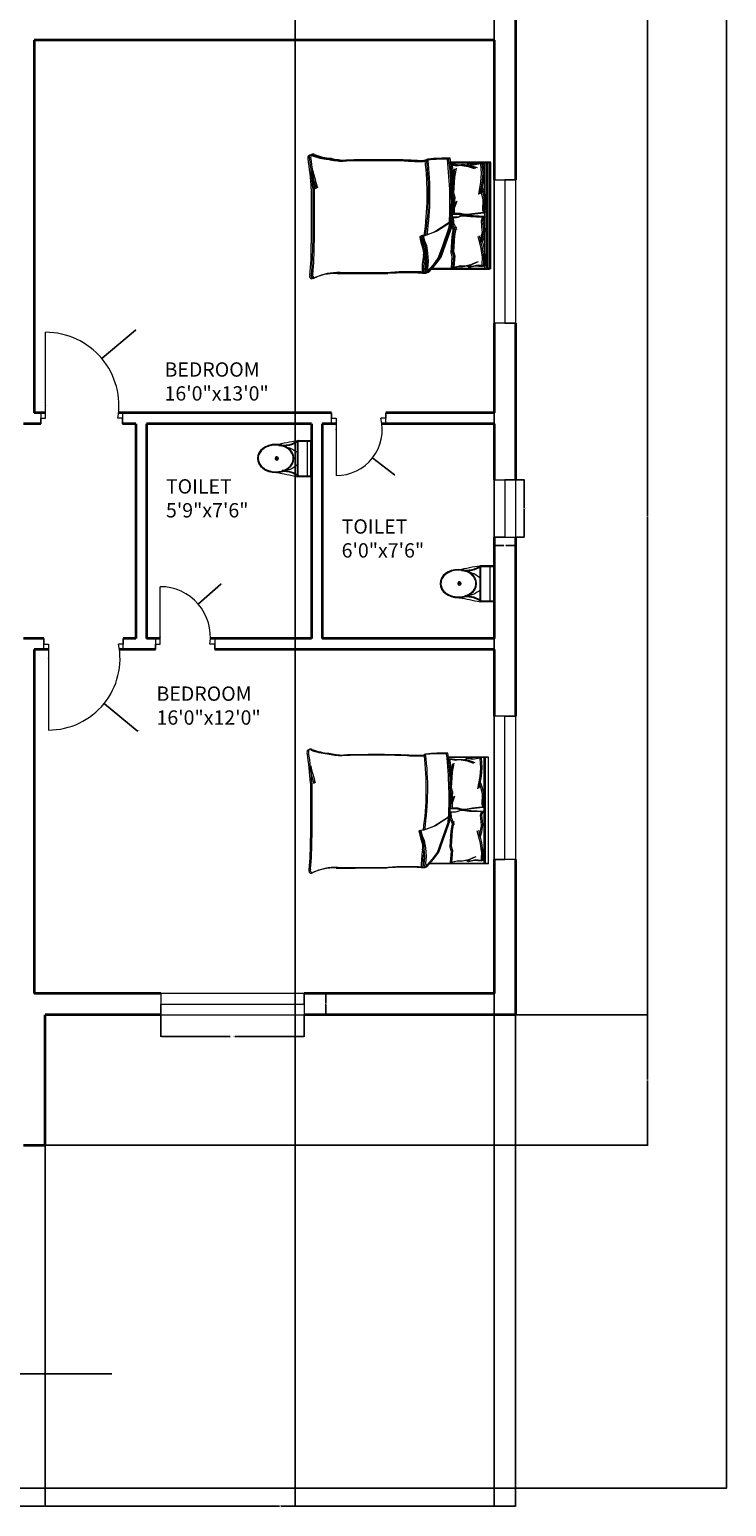
# Model space of a CAD drawing. Units: inches. Extents: x 1902 to 2626, y 1199 to 2408.
# Tile 5 of 9: x 2334 to 2626, y 1199 to 1817. Entities that reach past the tile are written whole.
import ezdxf

# ---------------------------------------------------------------- set-up
doc = ezdxf.new("R2010")
doc.units = ezdxf.units.IN
for name, color, linetype, lineweight in [('A-ANNO-DIMS', 2, 'Continuous', 18), ('A-ANNO-TTLB', 7, 'Continuous', 25), ('A-AREA-IDEN', 7, 'Continuous', 18), ('A-DOOR', 31, 'Continuous', 18), ('A-FLOR-FIXT', 9, 'Continuous', 18), ('A-FURN', 8, 'Continuous', 13), ('A-GLAZ', 181, 'Continuous', 18), ('A-WALL', 7, 'Continuous', 35)]:
    doc.layers.add(name, color=color, linetype=linetype, lineweight=lineweight)
doc.styles.get("Standard").update_dxf_attribs({"font": 'arial.ttf'})
doc.dimstyles.get("Standard").update_dxf_attribs({"dimtxt": 0.18, "dimasz": 0.18, "dimexe": 0.18, "dimexo": 0.0625, "dimgap": 0.09, "dimtad": 0, "dimtih": 1, "dimtoh": 1, "dimdec": 4, "dimzin": 0, "dimdsep": 46, "dimtxsty": 'Standard', "dimcen": 0.09, "dimadec": 0, "dimazin": 0, "dimtfac": 1, "dimtdec": 4, "dimtofl": 0, "dimtmove": 0, "dimatfit": 3, "dimfxl": 1, "dimtolj": 1, "dimtzin": 0, "dimarcsym": 0})

# ---------------------------------------------------------------- blocks, each defined once
blk = doc.blocks.new('A$C31115884')
for p, q in [((283, 498), (223, 498)), ((258, 466), (258, 523)), ((0, 200), (0, 0)), ((520, 200), (0, 200)), ((510, 54), (0, 54)), ((10, 190), (10, 10)), ((510, 190), (10, 190)), ((10, 10), (510, 10)), ((510, 10), (510, 190)), ((520, 0), (520, 200)), ((0, 0), (520, 0))]:
    blk.add_line(p, q)
blk.add_circle((256, 496), 23.6)
for centre, radius, start, end in [((2778, -205), 2807, 165.4549, 171.7133), ((-295, 403), 365, 324.2091, 9.3499), ((-295, 403), 375, 324.2091, 9.3499), ((806, 403), 365, 170.6501, 215.7909), ((3237, 905), 2807, 188.2867, 194.5451), ((384, 406), 293, 190.2774, 224.1564), ((139, 406), 293, 315.8436, 2.6563), ((806, 403), 375, 179.2036, 215.7909)]:
    blk.add_arc(centre, radius, start, end)
blk.add_ellipse((256, 510), major_axis=(0, -261), ratio=0.772727)
blk.add_open_spline([(256, 259), (263, 259), (270, 260), (288, 262), (299, 265), (320, 273), (330, 278), (350, 291), (360, 299), (378, 316), (386, 326), (402, 347), (409, 358), (421, 383), (427, 395), (436, 422), (440, 436), (445, 465), (447, 480), (448, 509), (448, 524), (445, 553), (443, 568), (436, 596), (432, 610), (422, 636), (416, 649), (402, 672), (395, 683), (379, 703), (370, 712), (351, 728), (341, 735), (321, 746), (310, 751), (289, 757), (278, 759), (256, 761), (245, 761), (223, 757), (212, 754), (191, 746), (181, 741), (161, 728), (151, 720), (133, 703), (125, 693), (110, 672), (103, 660), (90, 636), (85, 623), (76, 596), (72, 582), (67, 553), (66, 538), (64, 509), (65, 494), (68, 465), (70, 450), (77, 422), (81, 408), (91, 382), (97, 370), (111, 346), (118, 335), (135, 316), (144, 307), (162, 291), (172, 284), (193, 273), (203, 269), (225, 262), (236, 260), (250, 259), (253, 259), (256, 259)], degree=3, knots=[0, 0, 0, 0, 0.110105, 0.110105, 0.285049, 0.285049, 0.459994, 0.459994, 0.634938, 0.634938, 0.809882, 0.809882, 0.984827, 0.984827, 1.159771, 1.159771, 1.334715, 1.334715, 1.50966, 1.50966, 1.684604, 1.684604, 1.859549, 1.859549, 2.034493, 2.034493, 2.209437, 2.209437, 2.384382, 2.384382, 2.559326, 2.559326, 2.73427, 2.73427, 2.909215, 2.909215, 3.084159, 3.084159, 3.259103, 3.259103, 3.434048, 3.434048, 3.608992, 3.608992, 3.783936, 3.783936, 3.958881, 3.958881, 4.133825, 4.133825, 4.30877, 4.30877, 4.483714, 4.483714, 4.658658, 4.658658, 4.833603, 4.833603, 5.008547, 5.008547, 5.183491, 5.183491, 5.358436, 5.358436, 5.53338, 5.53338, 5.708324, 5.708324, 5.883269, 5.883269, 6.058213, 6.058213, 6.233158, 6.233158, 6.283185, 6.283185, 6.283185, 6.283185])
blk = doc.blocks.new('BED-DOUBLE')
for p, q in [((26.5, 49.58), (23.46, 46.12)), ((26.5, 49.58), (23.46, 46.12)), ((28.13, 49.66), (26.5, 49.58, 3.61)), ((28.13, 49.66), (26.5, 49.58, 3.61)), ((27.08, 48.15), (26.5, 49.58)), ((27.08, 48.15), (26.5, 49.58)), ((-0.01, 48.09), (0.59, 48.09)), ((-0.01, 48.09), (-0.01, 3.46)), ((-0.01, 47.87), (24.84, 47.87)), ((-0.01, 47.87), (24.84, 47.87)), ((0.59, 48.09), (25.44, 48.09)), ((0.59, 48.09), (25.44, 48.09)), ((1.43, 3.25), (1.43, 47.87)), ((1.43, 3.25), (1.43, 47.87)), ((2.02, 3.46), (2.02, 48.09)), ((2.02, 3.46), (2.02, 48.09)), ((2.38, 46.8), (2.29, 41.75)), ((2.38, 46.8), (2.29, 41.75)), ((2.38, 46.8), (5.38, 46.44)), ((2.38, 46.8), (5.38, 46.44)), ((2.98, 47.01), (2.89, 41.97)), ((2.98, 47.01), (2.89, 41.96)), ((2.98, 47.01), (5.98, 46.66)), ((2.98, 47.01), (5.98, 46.66)), ((7.7, 46.05), (5.2, 44.94)), ((7.7, 46.05), (5.2, 44.94)), ((5.38, 46.44), (7.78, 47)), ((5.38, 46.44), (7.78, 47)), ((8.3, 46.26), (5.8, 45.16)), ((8.3, 46.26), (5.8, 45.16)), ((5.98, 46.66), (8.38, 47.21)), ((5.98, 46.66), (8.38, 47.21)), ((11.04, 46.8), (7.7, 46.05)), ((11.04, 46.8), (7.7, 46.05)), ((7.78, 47), (8.76, 46.52)), ((7.78, 47), (8.76, 46.52)), ((11.64, 47.01), (8.3, 46.26)), ((11.64, 47.01), (8.3, 46.26)), ((8.38, 47.21), (9.35, 46.73)), ((8.38, 47.21), (9.35, 46.73)), ((12.54, 46.62), (11.04, 46.8)), ((12.54, 46.62), (11.04, 46.8)), ((13.14, 46.83), (11.64, 47.01)), ((13.14, 46.83), (11.64, 47.01)), ((15.47, 47.34), (12.54, 46.62)), ((15.47, 47.34), (12.54, 46.62)), ((16.07, 47.56), (13.14, 46.83)), ((16.07, 47.56), (13.14, 46.83)), ((15.09, 42.55), (15.47, 47.34)), ((15.09, 42.55), (15.47, 47.34)), ((15.69, 42.77), (16.07, 47.56)), ((15.69, 42.77), (16.07, 47.56)), ((21.44, 43.38), (19.56, 38.17)), ((21.44, 43.38), (19.56, 38.17)), ((22.87, 45.91), (20.84, 43.16)), ((22.87, 45.91), (20.84, 43.16)), ((23.46, 46.12), (21.44, 43.38)), ((23.46, 46.12), (21.44, 43.38)), ((25.9, 49.37), (22.87, 45.91)), ((25.9, 49.37), (22.87, 45.91)), ((27.53, 49.44), (25.9, 49.37, 3.61)), ((27.53, 49.44), (25.9, 49.37, 3.61)), ((26.48, 47.93), (25.9, 49.37)), ((26.48, 47.93), (25.9, 49.37)), ((26.19, 45.04), (26.48, 47.93)), ((26.19, 45.04), (26.48, 47.93)), ((26.48, 41.43), (26.19, 45.04)), ((26.48, 41.43), (26.19, 45.04)), ((26.79, 45.26), (27.08, 48.15)), ((26.79, 45.25), (27.08, 48.15)), ((27.08, 41.64), (26.79, 45.26)), ((27.08, 41.64), (26.79, 45.25)), ((2.29, 41.75), (2.37, 42.69)), ((2.29, 41.75), (2.37, 42.69)), ((2.37, 42.69), (2.86, 39.14)), ((2.37, 42.69), (2.86, 39.14)), ((2.86, 39.14), (4.12, 34.08)), ((2.86, 39.14), (4.12, 34.08)), ((2.89, 41.97), (2.97, 42.9)), ((2.89, 41.96), (2.97, 42.9)), ((2.97, 42.9), (3.46, 39.36)), ((2.97, 42.9), (3.46, 39.35)), ((3.46, 39.36), (4.72, 34.29)), ((3.46, 39.35), (4.72, 34.29)), ((15.61, 40.72), (15.09, 42.55)), ((15.61, 40.72), (15.09, 42.55)), ((15.21, 34.18), (15.61, 40.72)), ((15.21, 34.18), (15.61, 40.72)), ((16.21, 40.93), (15.69, 42.77)), ((16.21, 40.93), (15.69, 42.77)), ((15.81, 34.39), (16.21, 40.93)), ((15.81, 34.39), (16.21, 40.93)), ((18.97, 37.96), (16.23, 30.17)), ((18.97, 37.96), (16.23, 30.17)), ((19.56, 38.17), (16.82, 30.38)), ((19.56, 38.17), (16.82, 30.38)), ((20.84, 43.16), (18.97, 37.96)), ((20.84, 43.16), (18.97, 37.96)), ((26.91, 38.25), (26.48, 41.43)), ((26.91, 38.24), (26.48, 41.43)), ((27.78, 36.37), (26.91, 38.25)), ((27.78, 36.36), (26.91, 38.24)), ((27.51, 38.46), (27.08, 41.64)), ((27.51, 38.46), (27.08, 41.64)), ((28.38, 36.58), (27.51, 38.46)), ((28.38, 36.58), (27.51, 38.46)), ((74.59, 14.28), (74.59, 37.27)), ((74.59, 14.28), (74.59, 37.27)), ((2.87, 34.68), (2.36, 31.94)), ((2.87, 34.68), (2.36, 31.94)), ((2.36, 31.94), (2.38, 31.64)), ((2.36, 31.94), (2.38, 31.64)), ((2.38, 31.64), (2.78, 27.51)), ((2.38, 31.64), (2.78, 27.51)), ((3.42, 36.61), (2.87, 34.68)), ((3.42, 36.61), (2.87, 34.68)), ((3.47, 34.89), (2.96, 32.16)), ((3.47, 34.89), (2.96, 32.16)), ((2.96, 32.16), (2.98, 31.86)), ((2.96, 32.16), (2.98, 31.86)), ((2.98, 31.86), (3.37, 27.72)), ((2.98, 31.86), (3.37, 27.72)), ((4.02, 36.82), (3.47, 34.89)), ((4.02, 36.82), (3.47, 34.89)), ((15.63, 28.72), (14.43, 31.58)), ((15.63, 28.72), (14.43, 31.58)), ((14.59, 30.41), (15.21, 34.18)), ((14.59, 30.41), (15.21, 34.18)), ((16.22, 28.93), (15.02, 31.8)), ((16.22, 28.93), (15.02, 31.8)), ((15.18, 30.62), (15.81, 34.39)), ((15.18, 30.62), (15.81, 34.39)), ((16.23, 28.26), (22.29, 32.17)), ((16.23, 28.26), (22.29, 32.17)), ((16.82, 28.47), (22.89, 32.38)), ((16.82, 28.47), (22.89, 32.38)), ((22.29, 32.17), (26.48, 33.76)), ((22.29, 32.17), (26.48, 33.76)), ((22.89, 32.38), (27.08, 33.98)), ((22.89, 32.38), (27.08, 33.98)), ((26.48, 33.76), (28.36, 34.05)), ((26.48, 33.76), (28.36, 34.05)), ((27.08, 33.98), (28.96, 34.26)), ((27.08, 33.98), (28.96, 34.26)), ((28.36, 34.05), (27.78, 36.37)), ((28.36, 34.05), (27.78, 36.36)), ((28.96, 34.26), (28.38, 36.58)), ((28.96, 34.26), (28.38, 36.58)), ((73.99, 14.07), (73.99, 37.05)), ((73.99, 14.07), (73.99, 37.05)), ((1.74, 24.27), (6.74, 24.81)), ((1.74, 24.27), (6.74, 24.81)), ((2.78, 27.51), (2.32, 26.13)), ((2.78, 27.51), (2.32, 26.13)), ((2.32, 26.13), (7.34, 25.9)), ((2.32, 26.13), (7.34, 25.9)), ((2.34, 24.48), (7.33, 25.02)), ((2.34, 24.48), (7.33, 25.02)), ((3.37, 27.72), (2.92, 26.34)), ((3.37, 27.72), (2.92, 26.34)), ((2.92, 26.34), (7.94, 26.11)), ((2.92, 26.34), (7.94, 26.11)), ((6.74, 24.81), (9.71, 25.35)), ((6.74, 24.81), (9.71, 25.35)), ((7.33, 25.02), (10.3, 25.56)), ((7.33, 25.02), (10.3, 25.56)), ((7.34, 25.9), (10.34, 25.55)), ((7.34, 25.9), (10.34, 25.55)), ((7.94, 26.11), (10.94, 25.76)), ((7.94, 26.11), (10.94, 25.76)), ((9.71, 25.35), (10.92, 25.35)), ((9.71, 25.35), (10.92, 25.35)), ((10.3, 25.56), (11.52, 25.56)), ((10.3, 25.56), (11.52, 25.56)), ((10.34, 25.55), (11.55, 25.62)), ((10.34, 25.55), (11.55, 25.62)), ((10.92, 25.35), (12.68, 24.81)), ((10.92, 25.35), (12.68, 24.81)), ((10.94, 25.76), (12.15, 25.84)), ((10.94, 25.76), (12.15, 25.84)), ((11.52, 25.56), (13.27, 25.02)), ((11.52, 25.56), (13.27, 25.02)), ((11.55, 25.62), (13.27, 26.27)), ((11.55, 25.62), (13.27, 26.27)), ((12.15, 25.84), (13.87, 26.48)), ((12.15, 25.84), (13.87, 26.48)), ((12.68, 24.81), (15.18, 24.81)), ((12.68, 24.81), (15.18, 24.81)), ((13.27, 26.27), (15.77, 26.43)), ((13.27, 26.27), (15.77, 26.43)), ((13.27, 25.02), (15.78, 25.02)), ((13.27, 25.02), (15.78, 25.02)), ((13.87, 26.48), (16.37, 26.64)), ((13.87, 26.48), (16.37, 26.64)), ((15.18, 24.81), (15.18, 22.51)), ((15.18, 24.81), (15.18, 22.51)), ((15.77, 26.43), (15.63, 28.72)), ((15.77, 26.43), (15.63, 28.72)), ((15.78, 25.02), (15.78, 22.72)), ((15.78, 25.02), (15.78, 22.72)), ((16.37, 26.64), (16.22, 28.93)), ((16.37, 26.64), (16.22, 28.93)), ((2.28, 22.92), (1.74, 24.27)), ((2.28, 22.92), (1.74, 24.27)), ((2.15, 18.76), (2.28, 22.92)), ((2.15, 18.76), (2.28, 22.92)), ((2.15, 18.46), (2.15, 18.76)), ((2.15, 18.46), (2.15, 18.76)), ((2.88, 23.13), (2.34, 24.48)), ((2.88, 23.13), (2.34, 24.48)), ((2.74, 18.98), (2.88, 23.13)), ((2.74, 18.98), (2.88, 23.13)), ((2.74, 18.68), (2.74, 18.98)), ((2.74, 18.68), (2.74, 18.98)), ((3.42, 15.98), (2.74, 18.68)), ((3.42, 15.98), (2.74, 18.68)), ((15.18, 22.51), (14.16, 19.57)), ((15.18, 22.51), (14.16, 19.57)), ((15.78, 22.72), (14.76, 19.79)), ((15.78, 22.72), (14.76, 19.79)), ((15.09, 18.1), (15.47, 22.9)), ((15.09, 18.1), (15.47, 22.9)), ((15.69, 18.32), (16.07, 23.11)), ((15.69, 18.32), (16.07, 23.11)), ((2.82, 15.76), (2.15, 18.46)), ((2.82, 15.76), (2.15, 18.46)), ((3.5, 13.88), (2.82, 15.76)), ((3.5, 13.87), (2.82, 15.76)), ((3.09, 11.31), (4.04, 16.44)), ((3.09, 11.31), (4.04, 16.44)), ((4.09, 14.09), (3.42, 15.98)), ((4.09, 14.09), (3.42, 15.98)), ((3.69, 11.52), (4.63, 16.65)), ((3.69, 11.52), (4.63, 16.65)), ((15.61, 16.27), (15.09, 18.1)), ((15.61, 16.27), (15.09, 18.1)), ((15.21, 9.73), (15.61, 16.27)), ((15.21, 9.73), (15.61, 16.27)), ((16.21, 16.49), (15.69, 18.32)), ((16.21, 16.49), (15.69, 18.32)), ((15.81, 9.94), (16.21, 16.49)), ((15.81, 9.94), (16.21, 16.49)), ((2.8, 7.64), (2.82, 7.74)), ((2.8, 7.64), (2.82, 7.74)), ((3.11, 3.64), (2.8, 7.64)), ((3.11, 3.64), (2.8, 7.64)), ((2.82, 7.74), (3.09, 11.31)), ((2.82, 7.74), (3.09, 11.31)), ((3.4, 7.86), (3.42, 7.95)), ((3.4, 7.86), (3.42, 7.95)), ((3.71, 3.86), (3.4, 7.86)), ((3.71, 3.86), (3.4, 7.86)), ((3.42, 7.95), (3.69, 11.52)), ((3.42, 7.95), (3.69, 11.52)), ((14.59, 5.96), (15.21, 9.73)), ((14.59, 5.96), (15.21, 9.73)), ((15.18, 6.18), (15.81, 9.94)), ((15.18, 6.18), (15.81, 9.94)), ((15.21, 9.73), (15.51, 8.67)), ((15.21, 9.73), (15.51, 8.67)), ((15.51, 8.67), (16.19, 3.91)), ((15.51, 8.67), (16.19, 3.91)), ((15.81, 9.94), (16.11, 8.88)), ((15.81, 9.94), (16.11, 8.88)), ((16.11, 8.88), (16.78, 4.12)), ((16.11, 8.88), (16.78, 4.12)), ((16.91, 3.25), (-0.01, 3.25)), ((16.91, 3.25), (-0.01, 3.25)), ((17.5, 3.46), (0.59, 3.46)), ((17.5, 3.46), (0.59, 3.46)), ((3.09, 3.64), (6.06, 4.18)), ((3.09, 3.64), (6.06, 4.18)), ((3.69, 3.85), (6.66, 4.39)), ((3.69, 3.85), (6.66, 4.39)), ((8.36, 4.72), (5.79, 5.67)), ((8.36, 4.72), (5.79, 5.67)), ((6.06, 4.18), (8.49, 3.78)), ((6.06, 4.18), (8.49, 3.78)), ((8.95, 4.93), (6.39, 5.88)), ((8.95, 4.93), (6.39, 5.88)), ((6.66, 4.39), (9.09, 3.99)), ((6.66, 4.39), (9.09, 3.99)), ((11.73, 4.18), (8.36, 4.72)), ((11.73, 4.18), (8.36, 4.72)), ((8.49, 3.78), (9.44, 4.32)), ((8.49, 3.78), (9.44, 4.32)), ((12.33, 4.39), (8.95, 4.93)), ((12.33, 4.39), (8.95, 4.93)), ((9.09, 3.99), (10.03, 4.53)), ((9.09, 3.99), (10.03, 4.53)), ((13.22, 4.45), (11.73, 4.18)), ((13.22, 4.45), (11.73, 4.18)), ((13.81, 4.66), (12.33, 4.39)), ((13.81, 4.66), (12.33, 4.39)), ((16.19, 3.91), (13.22, 4.45)), ((16.19, 3.91), (13.22, 4.45)), ((16.78, 4.12), (13.81, 4.66)), ((16.78, 4.12), (13.81, 4.66))]:
    blk.add_line(p, q)
for centre, radius, start, end in [((33.9, 170.19), 120.92, 266.97912, 273.83645), ((33.9, 170.19), 120.92, 266.97912, 273.83645), ((-5.62, 48.14), 33.79, 349.87628, 2.56571), ((-5.62, 48.14), 33.79, 349.87628, 2.56571), ((34.5, 170.41), 120.92, 266.97912, 273.83645), ((34.5, 170.41), 120.92, 266.97912, 273.83645), ((63.32, -4210.02), 4259.62, 90.00217, 90.28689), ((63.32, -4210.02), 4259.62, 90.00217, 90.28689), ((63.92, -4209.8), 4259.62, 90.00217, 90.28689), ((63.92, -4209.8), 4259.62, 90.00217, 90.28689), ((64.11, 71.12), 21.54, 267.47136, 296.46809), ((64.11, 71.12), 21.54, 267.47136, 296.46809), ((64.71, 71.33), 21.54, 267.47136, 296.46809), ((64.71, 71.33), 21.54, 267.47136, 296.46809), ((73.64, 50.81), 1.03, 332.65876, 86.02002), ((73.64, 50.81), 1.03, 332.65876, 86.02002), ((198.21, 38.43), 124.23, 174.4998, 180.63509), ((198.21, 38.43), 124.23, 174.4998, 180.63509), ((74.24, 51.02), 1.03, 332.65876, 86.02002), ((74.24, 51.02), 1.03, 332.65876, 86.02002), ((198.8, 38.64), 124.23, 174.4998, 180.63509), ((198.8, 38.64), 124.23, 174.4998, 180.63509), ((-6.22, 47.93), 33.79, 349.87628, 2.56571), ((-6.22, 47.93), 33.79, 349.87628, 2.56571), ((32.74, 40.85), 5.81, 168.6608, 203.73842), ((32.74, 40.85), 5.81, 168.6608, 203.73842), ((1.38, 29.09), 27.69, 10.66171, 19.88058), ((1.38, 29.09), 27.69, 10.66171, 19.88058), ((33.33, 41.06), 5.81, 168.6608, 203.73842), ((33.33, 41.06), 5.81, 168.6608, 203.73842), ((1.98, 29.31), 27.69, 10.66171, 19.88058), ((1.98, 29.31), 27.69, 10.66171, 19.88058), ((145.95, 16.58), 120.47, 171.78449, 186.90062), ((145.95, 16.58), 120.47, 171.78449, 186.90062), ((146.55, 16.8), 120.47, 171.78449, 186.90062), ((146.55, 16.8), 120.47, 171.78449, 186.90062), ((28.42, 34.21), 0.172, 250.24637, 1.13765), ((28.42, 34.21), 0.172, 250.24637, 1.13765), ((29.01, 34.43), 0.172, 250.24637, 1.13765), ((29.01, 34.43), 0.172, 250.24637, 1.13765), ((169.99, 19.95), 154.04, 176.08655, 186.78213), ((169.99, 19.95), 154.04, 176.08655, 186.78213), ((170.58, 20.16), 154.04, 176.08655, 186.78213), ((170.58, 20.16), 154.04, 176.08655, 186.78213), ((-22.15, -16.08), 99.41, 13.38322, 17.70533), ((-22.15, -16.08), 99.41, 13.38322, 17.70533), ((-21.55, -15.86), 99.41, 13.38322, 17.70533), ((-21.55, -15.86), 99.41, 13.38322, 17.70533), ((187.53, 20.01), 113.69, 182.99578, 189.40907), ((187.53, 20.01), 113.69, 182.99578, 189.40907), ((188.12, 20.22), 113.69, 182.99578, 189.40907), ((188.12, 20.22), 113.69, 182.99578, 189.40907), ((18.76, 79.52), 77.79, 268.72178, 275.60397), ((18.76, 79.52), 77.79, 268.72178, 275.60397), ((19.36, 79.74), 77.79, 268.72178, 275.60397), ((19.36, 79.74), 77.79, 268.72178, 275.60397), ((29.1, -156.22), 158.84, 88.4762, 91.00819), ((29.1, -156.22), 158.84, 88.4762, 91.00819), ((29.7, -156), 158.84, 88.4762, 91.00819), ((29.7, -156.01), 158.84, 88.4762, 91.00819), ((47.26, 452.71), 450.36, 268.22771, 271.71854), ((47.26, 452.71), 450.36, 268.22771, 271.71854), ((47.85, 452.92), 450.36, 268.22771, 271.71854), ((47.85, 452.92), 450.36, 268.22771, 271.71854), ((60.24, -25.11), 27.67, 76.06484, 88.91125), ((60.24, -25.11), 27.67, 76.06484, 88.91125), ((60.83, -24.9), 27.67, 76.06484, 88.91125), ((60.83, -24.9), 27.67, 76.06484, 88.91125), ((65.61, -20.22), 22, 67.97508, 86.652), ((65.61, -20.22), 22, 67.97508, 86.652), ((66.21, -20.01), 22, 67.97508, 86.652), ((66.21, -20.01), 22, 67.97508, 86.652), ((74.43, 1.02), 1.02, 236.17358, 23.47814), ((74.43, 1.02), 1.02, 236.17358, 23.47814), ((75.03, 1.23), 1.02, 236.17358, 23.47814), ((75.03, 1.23), 1.02, 236.17358, 23.47814)]:
    blk.add_arc(centre, radius, start, end)
blk = doc.blocks.new('WINDOW-60-A')
for p, q in [((0, 9), (0, 0)), ((60, 9), (0, 9)), ((60, 4.5), (60, 9)), ((60, 9), (60, 0)), ((0, 0), (0, 4.5)), ((0, 4.5), (60, 4.5)), ((0, 0), (60, 0))]:
    blk.add_line(p, q)
blk = doc.blocks.new('WINDOW-60-B')
for p, q in [((0, 60), (9, 60)), ((0, 60), (0, 0)), ((9, 60), (4.5, 60)), ((4.5, 60), (4.5, 0)), ((9, 60), (9, 0)), ((9, 0), (0, 0)), ((4.5, 0), (9, 0))]:
    blk.add_line(p, q)
blk = doc.blocks.new('WINDOW-24')
for p, q in [((0, 24), (9, 24)), ((0, 24), (0, 0)), ((9, 24), (4.5, 24)), ((4.5, 24), (4.5, 0)), ((9, 24), (9, 0)), ((4.5, 0), (0, 0)), ((0, 0), (9, 0))]:
    blk.add_line(p, q)
blk = doc.blocks.new('*D16')
at = {"layer": 'A-ANNO-DIMS', "color": 0, "lineweight": -2, "transparency": 16777216}
for p, q in [((2389.37, 1404.41), (2389.37, 1395.29)), ((2449.37, 1404.41), (2449.37, 1395.29)), ((2389.55, 1395.47), (2418.41, 1395.47)), ((2449.19, 1395.47), (2420.34, 1395.47))]:
    blk.add_line(p, q, dxfattribs=at)
at = {"layer": 'A-ANNO-DIMS', "color": 0, "transparency": 16777216}
for points in [[(2389.55, 1395.5), (2389.55, 1395.44), (2389.37, 1395.47)], [(2449.19, 1395.5), (2449.19, 1395.44), (2449.37, 1395.47)]]:
    blk.add_solid(points, dxfattribs=at)
at = {"layer": 'Defpoints', "color": 0, "transparency": 16777216}
for p in [(2389.37, 1404.47), (2449.37, 1404.47), (2449.37, 1395.47)]:
    blk.add_point(p, dxfattribs=at)
at = {"layer": 'A-ANNO-DIMS', "color": 0, "transparency": 16777216, "insert": (2419.37, 1395.47), "char_height": 0.18, "attachment_point": 5}
blk.add_mtext('\\A1;WIN. A 60 TYP.', dxfattribs=at)
blk = doc.blocks.new('*D17')
at = {"layer": 'A-ANNO-DIMS', "color": 0, "lineweight": -2, "transparency": 16777216}
for p, q in [((2449.44, 1413.47), (2458.55, 1413.47)), ((2458.37, 1413.29), (2458.37, 1409.16)), ((2449.44, 1404.47), (2458.55, 1404.47)), ((2458.37, 1404.65), (2458.37, 1408.79))]:
    blk.add_line(p, q, dxfattribs=at)
at = {"layer": 'A-ANNO-DIMS', "color": 0, "transparency": 16777216}
for points in [[(2458.34, 1413.29), (2458.4, 1413.29), (2458.37, 1413.47)], [(2458.34, 1404.65), (2458.4, 1404.65), (2458.37, 1404.47)]]:
    blk.add_solid(points, dxfattribs=at)
at = {"layer": 'Defpoints', "color": 0, "transparency": 16777216}
for p in [(2449.37, 1413.47), (2458.37, 1413.47), (2449.37, 1404.47)]:
    blk.add_point(p, dxfattribs=at)
at = {"layer": 'A-ANNO-DIMS', "color": 0, "transparency": 16777216, "insert": (2458.37, 1408.97), "char_height": 0.18, "attachment_point": 5}
blk.add_mtext('\\A1;9 TYP.', dxfattribs=at)
blk = doc.blocks.new('*D20')
at = {"layer": 'A-ANNO-DIMS', "color": 0, "lineweight": -2, "transparency": 16777216}
for p, q in [((2537.91, 1628.52), (2541.63, 1628.52)), ((2541.45, 1628.34), (2541.45, 1616.71)), ((2541.45, 1604.7), (2541.45, 1616.34)), ((2537.91, 1604.52), (2541.63, 1604.52))]:
    blk.add_line(p, q, dxfattribs=at)
at = {"layer": 'A-ANNO-DIMS', "color": 0, "transparency": 16777216}
for points in [[(2541.42, 1628.34), (2541.48, 1628.34), (2541.45, 1628.52)], [(2541.42, 1604.7), (2541.48, 1604.7), (2541.45, 1604.52)]]:
    blk.add_solid(points, dxfattribs=at)
at = {"layer": 'Defpoints', "color": 0, "transparency": 16777216}
for p in [(2537.85, 1628.52), (2541.45, 1628.52), (2537.85, 1604.52)]:
    blk.add_point(p, dxfattribs=at)
at = {"layer": 'A-ANNO-DIMS', "color": 0, "transparency": 16777216, "insert": (2541.45, 1616.52), "char_height": 0.18, "attachment_point": 5}
blk.add_mtext('\\A1;WIN. C 24 TYP.', dxfattribs=at)
blk = doc.blocks.new('*D21')
at = {"layer": 'A-ANNO-DIMS', "color": 0, "lineweight": -2, "transparency": 16777216}
for p, q in [((2528.85, 1604.46), (2528.85, 1600.74)), ((2537.85, 1604.46), (2537.85, 1600.74)), ((2529.03, 1600.92), (2532.89, 1600.92)), ((2537.67, 1600.92), (2533.81, 1600.92))]:
    blk.add_line(p, q, dxfattribs=at)
at = {"layer": 'A-ANNO-DIMS', "color": 0, "transparency": 16777216}
for points in [[(2529.03, 1600.95), (2529.03, 1600.89), (2528.85, 1600.92)], [(2537.67, 1600.95), (2537.67, 1600.89), (2537.85, 1600.92)]]:
    blk.add_solid(points, dxfattribs=at)
at = {"layer": 'Defpoints', "color": 0, "transparency": 16777216}
for p in [(2528.85, 1604.52), (2537.85, 1604.52), (2537.85, 1600.92)]:
    blk.add_point(p, dxfattribs=at)
at = {"layer": 'A-ANNO-DIMS', "color": 0, "transparency": 16777216, "insert": (2533.35, 1600.92), "char_height": 0.18, "attachment_point": 5}
blk.add_mtext('\\A1;9 TYP.', dxfattribs=at)
blk = doc.blocks.new('*D31')
at = {"layer": 'A-ANNO-DIMS', "color": 0, "lineweight": -2, "transparency": 16777216}
for p, q in [((2202.85, 1349.87), (2202.85, 1198.67)), ((2340.85, 1349.87), (2340.85, 1198.67)), ((2203.03, 1198.85), (2271.57, 1198.85)), ((2340.67, 1198.85), (2272.13, 1198.85))]:
    blk.add_line(p, q, dxfattribs=at)
at = {"layer": 'A-ANNO-DIMS', "color": 0, "transparency": 16777216}
for points in [[(2203.03, 1198.88), (2203.03, 1198.82), (2202.85, 1198.85)], [(2340.67, 1198.88), (2340.67, 1198.82), (2340.85, 1198.85)]]:
    blk.add_solid(points, dxfattribs=at)
at = {"layer": 'Defpoints', "color": 0, "transparency": 16777216}
for p in [(2202.85, 1349.93), (2340.85, 1349.93), (2340.85, 1198.85)]:
    blk.add_point(p, dxfattribs=at)
at = {"layer": 'A-ANNO-DIMS', "color": 0, "transparency": 16777216, "insert": (2271.85, 1198.85), "char_height": 0.18, "attachment_point": 5}
blk.add_mtext('\\A1;138', dxfattribs=at)
blk = doc.blocks.new('*D32')
at = {"layer": 'A-ANNO-DIMS', "color": 0, "lineweight": -2, "transparency": 16777216}
for p, q in [((2537.85, 1404.41), (2537.85, 1198.67)), ((2340.85, 1349.87), (2340.85, 1198.67)), ((2341.03, 1198.85), (2439.07, 1198.85)), ((2537.67, 1198.85), (2439.63, 1198.85))]:
    blk.add_line(p, q, dxfattribs=at)
at = {"layer": 'A-ANNO-DIMS', "color": 0, "transparency": 16777216}
for points in [[(2341.03, 1198.88), (2341.03, 1198.82), (2340.85, 1198.85)], [(2537.67, 1198.88), (2537.67, 1198.82), (2537.85, 1198.85)]]:
    blk.add_solid(points, dxfattribs=at)
at = {"layer": 'Defpoints', "color": 0, "transparency": 16777216}
for p in [(2537.85, 1404.47), (2340.85, 1349.93), (2537.85, 1198.85)]:
    blk.add_point(p, dxfattribs=at)
at = {"layer": 'A-ANNO-DIMS', "color": 0, "transparency": 16777216, "insert": (2439.35, 1198.85), "char_height": 0.18, "attachment_point": 5}
blk.add_mtext('\\A1;197', dxfattribs=at)
blk = doc.blocks.new('*D34')
at = {"layer": 'A-ANNO-DIMS', "color": 0, "lineweight": -2, "transparency": 16777216}
for p, q in [((2528.91, 1821.47), (2593.33, 1821.47)), ((2593.15, 1821.29), (2593.15, 1613.15)), ((2593.15, 1404.65), (2593.15, 1612.79)), ((2537.91, 1404.47), (2593.33, 1404.47))]:
    blk.add_line(p, q, dxfattribs=at)
at = {"layer": 'A-ANNO-DIMS', "color": 0, "transparency": 16777216}
for points in [[(2593.12, 1821.29), (2593.18, 1821.29), (2593.15, 1821.47)], [(2593.12, 1404.65), (2593.18, 1404.65), (2593.15, 1404.47)]]:
    blk.add_solid(points, dxfattribs=at)
at = {"layer": 'Defpoints', "color": 0, "transparency": 16777216}
for p in [(2528.85, 1821.47), (2593.15, 1821.47), (2537.85, 1404.47)]:
    blk.add_point(p, dxfattribs=at)
at = {"layer": 'A-ANNO-DIMS', "color": 0, "transparency": 16777216, "insert": (2593.15, 1612.97), "char_height": 0.18, "attachment_point": 5}
blk.add_mtext('\\A1;417', dxfattribs=at)
blk = doc.blocks.new('*D36')
at = {"layer": 'A-ANNO-DIMS', "color": 0, "lineweight": -2, "transparency": 16777216}
for p, q in [((2537.91, 1404.47), (2593.33, 1404.47)), ((2593.15, 1404.29), (2593.15, 1377.38)), ((2593.15, 1350.11), (2593.15, 1377.02)), ((2340.91, 1349.93), (2593.33, 1349.93))]:
    blk.add_line(p, q, dxfattribs=at)
at = {"layer": 'A-ANNO-DIMS', "color": 0, "transparency": 16777216}
for points in [[(2593.12, 1404.29), (2593.18, 1404.29), (2593.15, 1404.47)], [(2593.12, 1350.11), (2593.18, 1350.11), (2593.15, 1349.93)]]:
    blk.add_solid(points, dxfattribs=at)
at = {"layer": 'Defpoints', "color": 0, "transparency": 16777216}
for p in [(2537.85, 1404.47), (2593.15, 1404.47), (2340.85, 1349.93)]:
    blk.add_point(p, dxfattribs=at)
at = {"layer": 'A-ANNO-DIMS', "color": 0, "transparency": 16777216, "insert": (2593.15, 1377.2), "char_height": 0.18, "attachment_point": 5}
blk.add_mtext('\\A1;54.54', dxfattribs=at)
blk = doc.blocks.new('*D37')
at = {"layer": 'A-ANNO-DIMS', "color": 0, "lineweight": -2, "transparency": 16777216}
for p, q in [((2445.52, 2280.41), (2445.52, 1198.67)), ((2528.85, 2280.41), (2528.85, 1198.67)), ((2445.7, 1198.85), (2486.79, 1198.85)), ((2528.67, 1198.85), (2487.58, 1198.85))]:
    blk.add_line(p, q, dxfattribs=at)
at = {"layer": 'A-ANNO-DIMS', "color": 0, "transparency": 16777216}
for points in [[(2445.7, 1198.88), (2445.7, 1198.82), (2445.52, 1198.85)], [(2528.67, 1198.88), (2528.67, 1198.82), (2528.85, 1198.85)]]:
    blk.add_solid(points, dxfattribs=at)
at = {"layer": 'Defpoints', "color": 0, "transparency": 16777216}
for p in [(2445.52, 2280.47), (2528.85, 2280.47), (2528.85, 1198.85)]:
    blk.add_point(p, dxfattribs=at)
at = {"layer": 'A-ANNO-DIMS', "color": 0, "transparency": 16777216, "insert": (2487.18, 1198.85), "char_height": 0.18, "attachment_point": 5}
blk.add_mtext('\\A1;83.33', dxfattribs=at)
blk = doc.blocks.new('*D47')
at = {"layer": 'A-ANNO-DIMS', "color": 0, "lineweight": -2, "transparency": 16777216}
for p, q in [((2378.7, 1691.12), (2364.73, 1679.38)), ((2378.88, 1691.12), (2378.7, 1691.12)), ((2341, 1659.52), (2341.18, 1659.52)), ((2341.09, 1659.43), (2341.09, 1659.61))]:
    blk.add_line(p, q, dxfattribs=at)
at = {"layer": 'A-ANNO-DIMS', "color": 0, "transparency": 16777216}
blk.add_solid([(2364.71, 1679.41), (2364.75, 1679.36), (2364.59, 1679.27)], dxfattribs=at)
at = {"layer": 'Defpoints', "color": 0, "transparency": 16777216}
for p in [(2364.59, 1679.27), (2341.09, 1659.52)]:
    blk.add_point(p, dxfattribs=at)
at = {"layer": 'A-ANNO-DIMS', "color": 0, "transparency": 16777216, "insert": (2379.29, 1691.12), "char_height": 0.18, "attachment_point": 5}
blk.add_mtext('\\A1;R30.7', dxfattribs=at)
blk = doc.blocks.new('*D48')
at = {"layer": 'A-ANNO-DIMS', "color": 0, "lineweight": -2, "transparency": 16777216}
for p, q in [((2342.25, 1553.63), (2342.43, 1553.63)), ((2342.34, 1553.54), (2342.34, 1553.72)), ((2379.46, 1523.44), (2365.68, 1534.65)), ((2379.64, 1523.44), (2379.46, 1523.44))]:
    blk.add_line(p, q, dxfattribs=at)
at = {"layer": 'A-ANNO-DIMS', "color": 0, "transparency": 16777216}
blk.add_solid([(2365.7, 1534.67), (2365.66, 1534.62), (2365.54, 1534.76)], dxfattribs=at)
at = {"layer": 'Defpoints', "color": 0, "transparency": 16777216}
for p in [(2342.34, 1553.63), (2365.54, 1534.76)]:
    blk.add_point(p, dxfattribs=at)
at = {"layer": 'A-ANNO-DIMS', "color": 0, "transparency": 16777216, "insert": (2380.19, 1523.44), "char_height": 0.18, "attachment_point": 5}
blk.add_mtext('\\A1;R29.906', dxfattribs=at)
blk = doc.blocks.new('*D53')
at = {"layer": 'A-ANNO-DIMS', "color": 0, "lineweight": -2, "transparency": 16777216}
for p, q in [((2414.48, 1584.78), (2405.08, 1576.6)), ((2414.66, 1584.78), (2414.48, 1584.78)), ((2388.95, 1562.65), (2389.13, 1562.65)), ((2389.04, 1562.56), (2389.04, 1562.74))]:
    blk.add_line(p, q, dxfattribs=at)
at = {"layer": 'A-ANNO-DIMS', "color": 0, "transparency": 16777216}
blk.add_solid([(2405.06, 1576.62), (2405.1, 1576.57), (2404.94, 1576.48)], dxfattribs=at)
at = {"layer": 'Defpoints', "color": 0, "transparency": 16777216}
for p in [(2404.94, 1576.48), (2389.04, 1562.65)]:
    blk.add_point(p, dxfattribs=at)
at = {"layer": 'A-ANNO-DIMS', "color": 0, "transparency": 16777216, "insert": (2415.21, 1584.78), "char_height": 0.18, "attachment_point": 5}
blk.add_mtext('\\A1;R21.077', dxfattribs=at)
blk = doc.blocks.new('*D57')
at = {"layer": 'A-ANNO-DIMS', "color": 0, "lineweight": -2, "transparency": 16777216}
for p, q in [((2462.67, 1649.53), (2462.85, 1649.53)), ((2462.76, 1649.44), (2462.76, 1649.62)), ((2487.11, 1630.53), (2478.12, 1637.54)), ((2487.29, 1630.53), (2487.11, 1630.53))]:
    blk.add_line(p, q, dxfattribs=at)
at = {"layer": 'A-ANNO-DIMS', "color": 0, "transparency": 16777216}
blk.add_solid([(2478.14, 1637.57), (2478.1, 1637.52), (2477.97, 1637.65)], dxfattribs=at)
at = {"layer": 'Defpoints', "color": 0, "transparency": 16777216}
for p in [(2462.76, 1649.53), (2477.97, 1637.65)]:
    blk.add_point(p, dxfattribs=at)
at = {"layer": 'A-ANNO-DIMS', "color": 0, "transparency": 16777216, "insert": (2487.84, 1630.53), "char_height": 0.18, "attachment_point": 5}
blk.add_mtext('\\A1;R19.303', dxfattribs=at)

msp = doc.modelspace()

# ---------------------------------------------------------------- linework, layer by layer
at = {"layer": 'A-ANNO-TTLB'}
msp.add_line((2104.9287, 1254.1475), (2368.8083, 1254.1475), dxfattribs=at)
msp.add_lwpolyline([(1901.6928, 2408.1473), (2626.1646, 2408.1473), (2626.1646, 1206.3103), (1901.6928, 1206.3103)], close=True, dxfattribs=at)
at = {"layer": 'A-DOOR'}
for p, q in [((2341.0862, 1654.2233), (2341.0862, 1690.2233)), ((2339.0862, 1656.4733), (2339.0862, 1651.9733)), ((2339.0862, 1651.9733), (2339.0862, 1654.2233)), ((2339.0862, 1654.2233), (2341.0862, 1654.2233)), ((2339.0862, 1651.9733), (2339.0862, 1651.9733)), ((2373.3259, 1654.2233), (2371.3259, 1654.2233)), ((2373.3259, 1656.4733), (2373.3259, 1651.9733)), ((2373.3259, 1651.9733), (2373.3259, 1654.2233)), ((2460.7554, 1651.9733), (2460.7554, 1656.4733)), ((2460.7554, 1656.4733), (2460.7554, 1654.2233)), ((2460.7554, 1654.2233), (2460.7554, 1654.2233)), ((2460.7554, 1654.2233), (2462.7554, 1654.2233)), ((2462.7554, 1654.2233), (2462.7554, 1630.2233)), ((2483.4786, 1654.2233), (2481.4786, 1654.2233)), ((2483.4786, 1651.9733), (2483.4786, 1656.4733)), ((2483.4786, 1656.4733), (2483.4786, 1654.2233)), ((2389.0386, 1559.7233), (2389.0386, 1583.7233)), ((2340.3371, 1557.4733), (2340.3371, 1561.9733)), ((2340.3371, 1561.9733), (2340.3371, 1559.7233)), ((2340.3371, 1559.7233), (2342.3371, 1559.7233)), ((2342.3371, 1559.7233), (2342.3371, 1523.7233)), ((2373.6154, 1559.7233), (2371.6154, 1559.7233)), ((2373.6154, 1557.4733), (2373.6154, 1561.9733)), ((2373.6154, 1561.9733), (2373.6154, 1559.7233)), ((2387.0386, 1561.9733), (2387.0386, 1557.4733)), ((2387.0386, 1557.4733), (2387.0386, 1559.7233)), ((2387.0386, 1559.7233), (2389.0386, 1559.7233)), ((2411.9122, 1559.7233), (2409.9122, 1559.7233)), ((2411.9122, 1561.9733), (2411.9122, 1557.4733)), ((2411.9122, 1557.4733), (2411.9122, 1559.7233))]:
    msp.add_line(p, q, dxfattribs=at)
for centre, radius, start, end in [((2341.0862, 1659.5228), 30.7005, 350.0598422, 90), ((2462.7554, 1649.5267), 19.3033, 270, 14.0818678), ((2389.0386, 1562.6461), 21.0772, 352.029104, 90), ((2342.3371, 1553.6292), 29.9058, 270, 11.7579684)]:
    msp.add_arc(centre, radius, start, end, dxfattribs=at)
at = {"layer": 'A-WALL'}
for p, q in [((2537.8507, 1865.0569), (2537.8507, 1754.0445)), ((2528.8507, 1812.4733), (2336.3507, 1812.4733)), ((2336.3507, 1812.4733), (2336.3507, 1656.4733)), ((2528.8507, 1812.4733), (2528.8507, 1754.0445)), ((2528.8507, 1694.0445), (2528.8507, 1656.4733)), ((2537.8507, 1694.0445), (2537.8507, 1628.5226)), ((2339.0862, 1651.9733), (2331.8507, 1651.9733)), ((2341.0862, 1656.4733), (2336.3507, 1656.4733)), ((2460.7554, 1656.4733), (2371.6349, 1656.4733)), ((2378.8507, 1651.9733), (2373.3259, 1651.9733)), ((2378.8507, 1651.9733), (2378.8507, 1561.9733)), ((2383.3507, 1651.9733), (2383.3507, 1561.9733)), ((2452.3507, 1651.9733), (2383.3507, 1651.9733)), ((2452.3507, 1651.9733), (2452.3507, 1561.9733)), ((2456.8507, 1651.9733), (2456.8507, 1561.9733)), ((2462.7554, 1651.9733), (2456.8507, 1651.9733)), ((2528.8507, 1651.9733), (2481.903, 1651.9733)), ((2528.8507, 1656.4733), (2483.4786, 1656.4733)), ((2528.8507, 1651.9733), (2528.8507, 1628.5226)), ((2528.8507, 1604.5226), (2528.8507, 1561.9733)), ((2537.8507, 1604.5226), (2537.8507, 1529.5415)), ((2340.3371, 1561.9733), (2331.8507, 1561.9733)), ((2378.8507, 1561.9733), (2373.6154, 1561.9733)), ((2389.0386, 1561.9733), (2383.3507, 1561.9733)), ((2452.3507, 1561.9733), (2410.1051, 1561.9733)), ((2528.8507, 1561.9733), (2456.8507, 1561.9733)), ((2336.3507, 1557.4733), (2336.3507, 1413.4733)), ((2342.3371, 1557.4733), (2336.3507, 1557.4733)), ((2387.0386, 1557.4733), (2371.9949, 1557.4733)), ((2528.8507, 1557.4733), (2411.9122, 1557.4733)), ((2528.8507, 1557.4733), (2528.8507, 1529.5415)), ((2528.8507, 1469.5415), (2528.8507, 1413.4733)), ((2537.8507, 1469.5415), (2537.8507, 1404.4733)), ((2389.3745, 1413.4733), (2336.3507, 1413.4733)), ((2528.8507, 1413.4733), (2449.3745, 1413.4733)), ((2340.8507, 1349.9322), (2340.8507, 1404.4733)), ((2389.3745, 1404.4733), (2340.8507, 1404.4733)), ((2537.8507, 1404.4733), (2449.3745, 1404.4733)), ((2331.8507, 1349.9322), (2340.8507, 1349.9322))]:
    msp.add_line(p, q, dxfattribs=at)

# ---------------------------------------------------------------- block references
at = {"layer": 'A-FLOR-FIXT', "xscale": -0.0292470664339069, "yscale": 0.0292470664339069, "zscale": 0.0292470664339069, "rotation": 90}
for p in [(2452.3507, 1644.934), (2528.8507, 1592.532)]:
    msp.add_blockref('A$C31115884', p, dxfattribs=at)
at = {"layer": 'A-FURN', "rotation": 180}
for p in [(2526.9159, 1764.6213), (2527.5128, 1764.8346), (2526.5682, 1515.7678)]:
    msp.add_blockref('BED-DOUBLE', p, dxfattribs=at)
at = {"layer": 'A-GLAZ'}
for name, p in [('WINDOW-60-B', (2528.85, 1694.0481)), ('WINDOW-24', (2528.85, 1604.5206)), ('WINDOW-60-A', (2389.3784, 1404.47))]:
    msp.add_blockref(name, p, dxfattribs=at)
at = {"layer": 'A-GLAZ', "extrusion": (0, 0, -1), "zscale": -1, "rotation": 90}
msp.add_blockref('WINDOW-60-A', (-2528.8474, 1469.5455), dxfattribs=at)

# ---------------------------------------------------------------- texts
at = {"layer": 'A-AREA-IDEN', "char_height": 6, "attachment_point": 1}
for s, width, insert in [('BEDROOM\\P16\'0"x13\'0"', 184.89189, (2390.8776, 1677.6458)), ('TOILET\\P5\'9"x7\'6"', 112.798142, (2391.4754, 1628.718)), ('TOILET\\P6\'0"x7\'6"', 130.929034, (2465.0346, 1611.9286)), ('BEDROOM\\P16\'0"x12\'0"', 167.377087, (2387.509, 1541.9471))]:
    msp.add_mtext_dynamic_manual_height_columns(s, width=width, gutter_width=12.5, heights=[0], dxfattribs=dict(at, insert=insert))

# ---------------------------------------------------------------- dimensions: what is measured, and where the dimension line sits
at = {"layer": 'A-ANNO-DIMS'}
for base, p1, p2, override, picture, middle in [((2528.8507, 1198.8475), (2445.516, 2280.4733), (2528.8507, 2280.4733), {"dimdec": 2, "dimlfac": 1, "dimrnd": 0, "dimzin": 0, "dimdsep": 46, "dimlunit": 2}, '*D37', (2487.1833, 1198.8475)), ((2537.8507, 1198.8475), (2340.8507, 1349.9322), (2537.8507, 1404.4733), {"dimdec": 0, "dimlfac": 1, "dimrnd": 0, "dimzin": 0, "dimdsep": 46, "dimlunit": 2}, '*D32', (2439.3507, 1198.8475)), ((2340.8507, 1198.8475), (2202.8507, 1349.9322), (2340.8507, 1349.9322), {"dimdec": 0, "dimlfac": 1, "dimrnd": 0, "dimzin": 0, "dimdsep": 46, "dimlunit": 2}, '*D31', (2271.8507, 1198.8475))]:
    dim = msp.add_linear_dim(base=base, p1=p1, p2=p2, dimstyle='Standard', override=override, dxfattribs=at)
    dim.commit()
    dim.dimension.update_dxf_attribs({"geometry": picture, "text_midpoint": middle})
for base, p1, p2, override, picture, middle in [((2593.1507, 1821.4733), (2537.8507, 1404.4733), (2528.8507, 1821.4733), {"dimdec": 0, "dimlfac": 1, "dimrnd": 0, "dimzin": 0, "dimdsep": 46, "dimlunit": 2}, '*D34', (2593.1507, 1612.9733)), ((2593.1507, 1404.4733), (2340.8507, 1349.9322), (2537.8507, 1404.4733), {"dimdec": 2, "dimlfac": 1, "dimrnd": 0, "dimzin": 0, "dimdsep": 46, "dimlunit": 2}, '*D36', (2593.1507, 1377.2028))]:
    dim = msp.add_linear_dim(base=base, p1=p1, p2=p2, angle=90, dimstyle='Standard', override=override, dxfattribs=at)
    dim.commit()
    dim.dimension.update_dxf_attribs({"geometry": picture, "text_midpoint": middle})
for center, mpoint, override, picture, middle in [((2341.0862, 1659.5228), (2364.5939, 1679.2689), {"dimdec": 1, "dimlfac": 1, "dimrnd": 0, "dimzin": 0, "dimdsep": 46, "dimlunit": 2}, '*D47', (2379.2885, 1691.1166)), ((2462.7554, 1649.5267), (2477.975, 1637.653), {"dimdec": 3, "dimlfac": 1, "dimrnd": 0, "dimzin": 0, "dimdsep": 46, "dimlunit": 2}, '*D57', (2487.8365, 1630.5289)), ((2389.0386, 1562.6461), (2404.9422, 1576.4782), {"dimdec": 3, "dimlfac": 1, "dimrnd": 0, "dimzin": 0, "dimdsep": 46, "dimlunit": 2}, '*D53', (2415.2141, 1584.7774)), ((2342.3371, 1553.6292), (2365.5388, 1534.7601), {"dimdec": 3, "dimlfac": 1, "dimrnd": 0, "dimzin": 0, "dimdsep": 46, "dimlunit": 2}, '*D48', (2380.1896, 1523.4387))]:
    dim = msp.add_radius_dim(center=center, mpoint=mpoint, dimstyle='Standard', override=override, dxfattribs=at)
    dim.commit()
    dim.dimension.update_dxf_attribs({"geometry": picture, "text_midpoint": middle, "dimtype": 164})
for base, p1, p2, text, picture, middle in [((2541.4507, 1628.5226), (2537.8507, 1604.5226), (2537.8507, 1628.5226), 'WIN. C <> TYP.', '*D20', (2541.4507, 1616.5226)), ((2458.3745, 1413.4733), (2449.3745, 1404.4733), (2449.3745, 1413.4733), '<> TYP.', '*D17', (2458.3745, 1408.9733))]:
    dim = msp.add_linear_dim(base=base, p1=p1, p2=p2, angle=90, text=text, dimstyle='Standard', override={"dimdec": 0, "dimlfac": 1, "dimrnd": 0, "dimzin": 0, "dimdsep": 46, "dimlunit": 2}, dxfattribs=at)
    dim.commit()
    dim.dimension.update_dxf_attribs({"geometry": picture, "text_midpoint": middle})
for base, p1, p2, text, picture, middle in [((2537.8507, 1600.9226), (2528.8507, 1604.5226), (2537.8507, 1604.5226), '<> TYP.', '*D21', (2533.3507, 1600.9226)), ((2449.3745, 1395.4733), (2389.3745, 1404.4733), (2449.3745, 1404.4733), 'WIN. A <> TYP.', '*D16', (2419.3745, 1395.4733))]:
    dim = msp.add_linear_dim(base=base, p1=p1, p2=p2, text=text, dimstyle='Standard', override={"dimdec": 0, "dimlfac": 1, "dimrnd": 0, "dimzin": 0, "dimdsep": 46, "dimlunit": 2}, dxfattribs=at)
    dim.commit()
    dim.dimension.update_dxf_attribs({"geometry": picture, "text_midpoint": middle})

doc.saveas('drawing.dxf')
